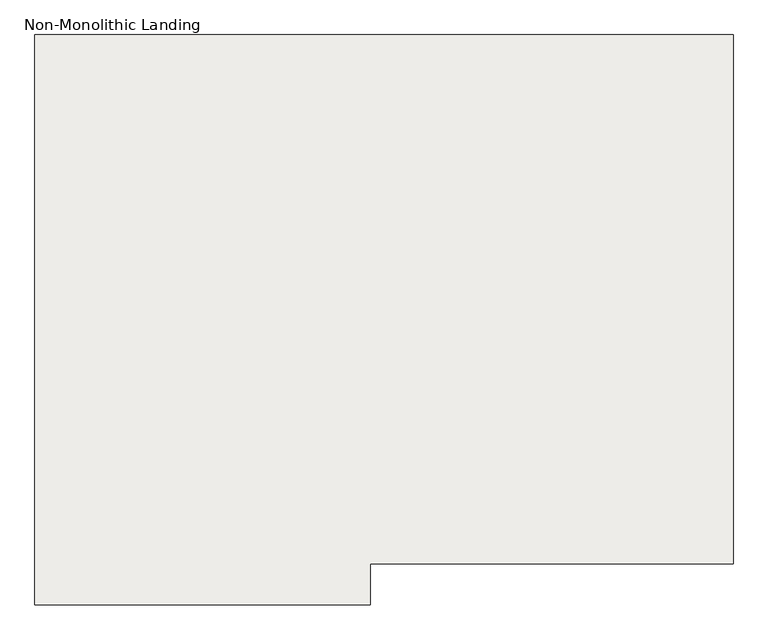
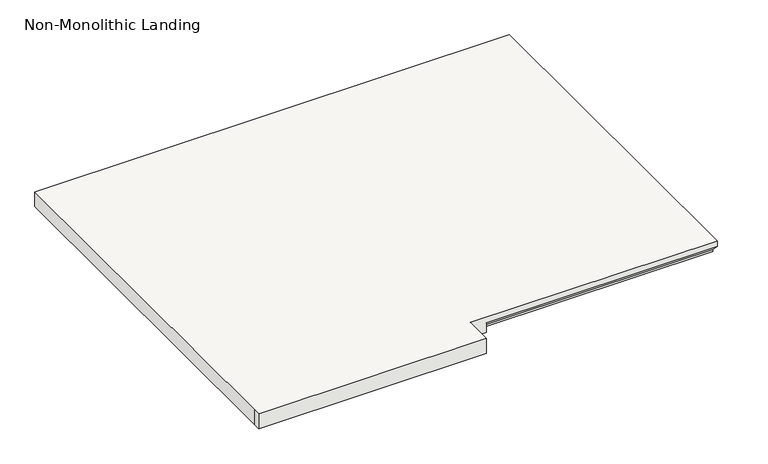
"""IFC4 building model written with IfcOpenShell, lengths in millimetres: slab geometry, Non-Monolithic Landing."""

from ifc_helpers import new_model, si_unit, origin, place, context, project, spatial, faceted_brep, source, transform, mapped, element, save


def non_monolithic_landing_20a8ff8f(model_context):
    return source(origin(), model_context, "Body", "Brep", [
        faceted_brep([(-5330.5155596, 6109.0076853, 7842.25), (-5330.5155596, 6083.6076853, 7867.65), (-6072.1955596, 6083.6076853, 7867.65), (-6072.1955596, 6109.0076853, 7842.25), (-5330.5155596, 7239.3076853, 7886.7), (-6854.5155596, 7239.3076853, 7886.7), (-6854.5155596, 6020.1076853, 7886.7), (-6854.5155596, 5994.7076853, 7886.7), (-6122.9955596, 5994.7076853, 7886.7), (-6122.9955596, 6020.1076853, 7886.7), (-6122.9955596, 6083.6076853, 7886.7), (-5330.5155596, 6083.6076853, 7886.7), (-6072.1955596, 6109.0076853, 7835.9), (-6072.1955596, 6083.6076853, 7835.9), (-6122.9955596, 6083.6076853, 7835.9), (-6122.9955596, 6020.1076853, 7835.9), (-6122.9955596, 5994.7076853, 7835.9), (-6854.5155596, 5994.7076853, 7835.9), (-6854.5155596, 6020.1076853, 7835.9), (-6854.5155596, 7239.3076853, 7835.9), (-5330.5155596, 7239.3076853, 7835.9), (-5330.5155596, 6109.0076853, 7835.9)], [[[0, 1, 2, 3]], [[4, 5, 6, 7, 8, 9, 10, 11]], [[12, 13, 14, 15, 16, 17, 18, 19, 20, 21]], [[13, 12, 3, 2]], [[12, 21, 0, 3]], [[4, 11, 1, 0, 21, 20]], [[5, 4, 20, 19]], [[6, 5, 19, 18]], [[7, 6, 18, 17]], [[8, 7, 17, 16]], [[9, 8, 16, 15]], [[10, 9, 15, 14]], [[11, 10, 14, 13, 2, 1]]]),
    ])


if __name__ == "__main__":
    model = new_model("IFC4")
    model_context = context("Model", 3, world=origin())
    ifc_project = project(units=[si_unit("LENGTHUNIT", "METRE", prefix="MILLI")], contexts=[model_context])
    site = spatial("IfcSite", under=ifc_project)
    building = spatial("IfcBuilding", under=site)
    placement = place(None, origin())
    non_monolithic_landing_shape = non_monolithic_landing_20a8ff8f(model_context)
    element("IfcSlab", 1, ObjectType="Non-Monolithic Landing", at=placement, inside=building, context=model_context, shape_type="MappedRepresentation", body=[
        mapped(non_monolithic_landing_shape, transform((0.0, 0.0, 0.0), x_axis=(1.0, 0.0, 0.0), y_axis=(0.0, 1.0, 0.0), z_axis=(0.0, 0.0, 1.0))),
    ])
    save(model, "model.ifc")
